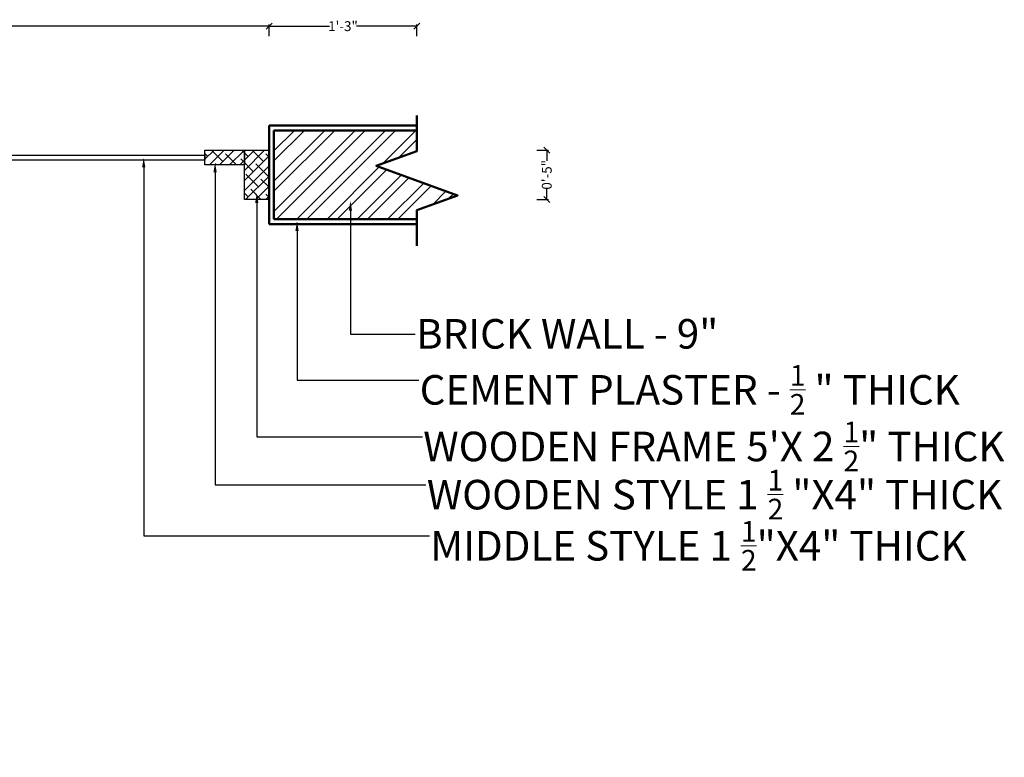
# Model space of a CAD drawing. Units: inches. Extents: x -54 to 163, y -154 to 48.
# Tile 2 of 3: x 30 to 129, y -154 to -79. Entities that reach past the tile are written whole.
import ezdxf
from ezdxf import colors
from ezdxf.entities.mleader import LeaderData, LeaderLine
from ezdxf.math import Vec2, Vec3

# ---------------------------------------------------------------- set-up
doc = ezdxf.new("R2010")
doc.units = ezdxf.units.IN
doc.header["$MEASUREMENT"] = 0
for name, color, linetype, lineweight in [('A-ANNO-DIMS', 2, 'Continuous', 18), ('A-ANNO-TEXT', 3, 'Continuous', 18), ('A-GLAZ', 4, 'Continuous', 25), ('A-GLAZ-PATT', 9, 'Continuous', 13), ('A-WALL', 7, 'Continuous', 50), ('A-WALL-PATT', 8, 'Continuous', 18)]:
    doc.layers.add(name, color=color, linetype=linetype, lineweight=lineweight)
doc.styles.get("Standard").update_dxf_attribs({"font": 'arial.ttf'})
doc.dimstyles.get("Standard").update_dxf_attribs({"dimtxt": 1, "dimasz": 0.6, "dimexe": 0.18, "dimexo": 0.0625, "dimgap": 0.09, "dimtad": 0, "dimdec": 1, "dimzin": 0, "dimdsep": 46, "dimlunit": 4, "dimtxsty": 'Standard', "dimblk": 'OBLIQUE', "dimcen": 0.09, "dimadec": 0, "dimazin": 0, "dimtfac": 1, "dimtdec": 1, "dimtofl": 0, "dimtmove": 0, "dimatfit": 3, "dimfxl": 1, "dimfxlon": 1, "dimtolj": 1, "dimtzin": 0, "dimarcsym": 0})

# ---------------------------------------------------------------- blocks, each defined once
blk = doc.blocks.new('_Oblique')
at = {"color": 0, "linetype": 'ByBlock', "lineweight": -2}
blk.add_line((-0.5, -0.5), (0.5, 0.5), dxfattribs=at)
blk = doc.blocks.new('*D34')
at = {"layer": 'A-ANNO-DIMS', "color": 0, "lineweight": -2, "transparency": 16777216}
for p, q in [((-24.085, -80.576), (-24.085, -79.396)), ((-24.085, -79.576), (13.993, -79.576)), ((54.915, -79.576), (16.837, -79.576)), ((54.915, -80.576), (54.915, -79.396))]:
    blk.add_line(p, q, dxfattribs=at)
at = {"layer": 'Defpoints', "color": 0, "transparency": 16777216}
for p in [(54.915, -79.576), (-24.085, -89.654), (54.915, -89.654)]:
    blk.add_point(p, dxfattribs=at)
at = {"layer": 'A-ANNO-DIMS', "color": 0, "lineweight": -2, "transparency": 16777216, "xscale": 0.6, "yscale": 0.6, "zscale": 0.6, "rotation": 180}
blk.add_blockref('_Oblique', (-24.085, -79.576), dxfattribs=at)
at = {"layer": 'A-ANNO-DIMS', "color": 0, "lineweight": -2, "transparency": 16777216, "xscale": 0.6, "yscale": 0.6, "zscale": 0.6}
blk.add_blockref('_Oblique', (54.915, -79.576), dxfattribs=at)
at = {"layer": 'A-ANNO-DIMS', "color": 0, "transparency": 16777216, "insert": (15.415, -79.576), "char_height": 1, "attachment_point": 5}
blk.add_mtext('\\A1;6\'-7"', dxfattribs=at)
blk = doc.blocks.new('*D35')
at = {"layer": 'A-ANNO-DIMS', "color": 0, "lineweight": -2, "transparency": 16777216}
for p, q in [((54.915, -80.576), (54.915, -79.396)), ((54.915, -79.576), (61.043, -79.576)), ((69.915, -79.576), (63.787, -79.576)), ((69.915, -80.576), (69.915, -79.396))]:
    blk.add_line(p, q, dxfattribs=at)
at = {"layer": 'Defpoints', "color": 0, "transparency": 16777216}
for p in [(69.915, -79.576), (54.915, -89.654), (69.915, -89.654)]:
    blk.add_point(p, dxfattribs=at)
at = {"layer": 'A-ANNO-DIMS', "color": 0, "lineweight": -2, "transparency": 16777216, "xscale": 0.6, "yscale": 0.6, "zscale": 0.6, "rotation": 180}
blk.add_blockref('_Oblique', (54.915, -79.576), dxfattribs=at)
at = {"layer": 'A-ANNO-DIMS', "color": 0, "lineweight": -2, "transparency": 16777216, "xscale": 0.6, "yscale": 0.6, "zscale": 0.6}
blk.add_blockref('_Oblique', (69.915, -79.576), dxfattribs=at)
at = {"layer": 'A-ANNO-DIMS', "color": 0, "transparency": 16777216, "insert": (62.415, -79.576), "char_height": 1, "attachment_point": 5}
blk.add_mtext('\\A1;1\'-3"', dxfattribs=at)
blk = doc.blocks.new('*D41')
at = {"layer": 'A-ANNO-DIMS', "color": 0, "lineweight": -2, "transparency": 16777216}
for p, q in [((-51.256, -89.654), (-52.436, -89.654)), ((-52.256, -89.654), (-52.256, -92.154)), ((-51.256, -92.154), (-52.436, -92.154)), ((-52.256, -92.154), (-52.256, -92.754))]:
    blk.add_line(p, q, dxfattribs=at)
at = {"layer": 'Defpoints', "color": 0, "transparency": 16777216}
for p in [(54.915, -89.654), (-52.256, -92.154), (52.415, -92.154)]:
    blk.add_point(p, dxfattribs=at)
at = {"layer": 'A-ANNO-DIMS', "color": 0, "lineweight": -2, "transparency": 16777216, "xscale": 0.6, "yscale": 0.6, "zscale": 0.6}
for p, rotation in [((-52.256, -89.654), 90), ((-52.256, -92.154), 270)]:
    blk.add_blockref('_Oblique', p, dxfattribs=dict(at, rotation=rotation))
at = {"layer": 'A-ANNO-DIMS', "color": 0, "transparency": 16777216, "insert": (-52.256, -95.339), "char_height": 1, "attachment_point": 5, "rotation": 90}
blk.add_mtext('\\A1;0\'-2 1/2"', dxfattribs=at)
blk = doc.blocks.new('*D42')
at = {"layer": 'A-ANNO-DIMS', "color": 0, "lineweight": -2, "transparency": 16777216}
for p, q in [((82.086, -92.154), (83.266, -92.154)), ((83.086, -92.154), (83.086, -93.235)), ((83.086, -97.154), (83.086, -96.073)), ((82.086, -97.154), (83.266, -97.154))]:
    blk.add_line(p, q, dxfattribs=at)
at = {"layer": 'Defpoints', "color": 0, "transparency": 16777216}
for p in [(-24.085, -92.154), (-24.085, -97.154), (83.086, -97.154)]:
    blk.add_point(p, dxfattribs=at)
at = {"layer": 'A-ANNO-DIMS', "color": 0, "lineweight": -2, "transparency": 16777216, "xscale": 0.6, "yscale": 0.6, "zscale": 0.6}
for p, rotation in [((83.086, -92.154), 90), ((83.086, -97.154), 270)]:
    blk.add_blockref('_Oblique', p, dxfattribs=dict(at, rotation=rotation))
at = {"layer": 'A-ANNO-DIMS', "color": 0, "transparency": 16777216, "insert": (83.086, -94.654), "char_height": 1, "attachment_point": 5, "rotation": 90}
blk.add_mtext('\\A1;0\'-5"', dxfattribs=at)

msp = doc.modelspace()

# ---------------------------------------------------------------- hatches: boundary and pattern name
at = {"layer": 'A-GLAZ-PATT'}
h = msp.add_hatch(dxfattribs=at)
h.set_pattern_fill('ANSI38', color=256, scale=5.8)
h.paths.add_polyline_path([(54.915, -92.154), (52.415, -92.154), (52.415, -97.154), (54.915, -97.154)])
h.paths.add_polyline_path([(52.415, -92.154), (48.415, -92.154), (48.415, -93.654), (52.415, -93.654)])
h.paths.add_polyline_path([(17.415, -92.154), (13.415, -92.154), (13.415, -93.654), (17.415, -93.654)])
h.paths.add_polyline_path([(-21.585, -92.154), (-24.085, -92.154), (-24.085, -97.154), (-21.585, -97.154)])
h.paths.add_polyline_path([(-17.585, -92.154), (-21.585, -92.154), (-21.585, -93.654), (-17.585, -93.654)])
at = {"layer": 'A-WALL-PATT'}
h = msp.add_hatch(dxfattribs=at)
h.set_pattern_fill('ANSI32', color=256, scale=5.8)
h.paths.add_polyline_path([(65.794, -93.742), (69.915, -92.242), (69.915, -90.154), (55.415, -90.154), (55.415, -99.154), (69.915, -99.154), (69.915, -98.242), (74.036, -96.742)])
h.paths.add_polyline_path([(-24.585, -90.154), (-39.085, -90.154), (-39.085, -92.242), (-34.964, -93.742), (-43.206, -96.742), (-39.085, -98.242), (-39.085, -99.154), (-24.585, -99.154)])

# ---------------------------------------------------------------- linework, layer by layer
at = {"layer": 'A-GLAZ'}
for points in [[(48.415, -92.654), (48.415, -93.154), (17.415, -93.154), (17.415, -92.654)], [(52.415, -92.154), (52.415, -93.654), (48.415, -93.654), (48.415, -92.154)], [(54.915, -92.154), (54.915, -97.154), (52.415, -97.154), (52.415, -92.154)]]:
    msp.add_lwpolyline(points, close=True, dxfattribs=at)
at = {"layer": 'A-WALL'}
for p, q in [((69.915, -89.654), (54.915, -89.654)), ((54.915, -89.654), (54.915, -99.654)), ((69.915, -90.154), (55.415, -90.154)), ((55.415, -90.154), (55.415, -99.154)), ((69.915, -99.654), (54.915, -99.654)), ((69.915, -99.154), (55.415, -99.154))]:
    msp.add_line(p, q, dxfattribs=at)
msp.add_lwpolyline([(69.915, -88.626), (69.915, -92.242), (65.794, -93.742), (74.036, -96.742), (69.915, -98.242), (69.915, -101.857)], dxfattribs=at)

# ---------------------------------------------------------------- dimensions: what is measured, and where the dimension line sits
at = {"layer": 'A-ANNO-DIMS'}
for base, p1, p2, picture, middle in [((54.915, -79.576), (-24.085, -89.654), (54.915, -89.654), '*D34', (15.415, -79.576)), ((69.915, -79.576), (54.915, -89.654), (69.915, -89.654), '*D35', (62.415, -79.576))]:
    dim = msp.add_linear_dim(base=base, p1=p1, p2=p2, dimstyle='Standard', override={"dimdec": 1, "dimlfac": 1, "dimrnd": 0, "dimzin": 1, "dimdsep": 46, "dimlunit": 4, "dimfrac": 2}, dxfattribs=at)
    dim.commit()
    dim.dimension.update_dxf_attribs({"geometry": picture, "text_midpoint": middle})
for base, p1, p2, picture, middle in [((-52.256, -92.154), (54.915, -89.654), (52.415, -92.154), '*D41', (-52.256, -95.339)), ((83.086, -97.154), (-24.085, -92.154), (-24.085, -97.154), '*D42', (83.086, -94.654))]:
    dim = msp.add_linear_dim(base=base, p1=p1, p2=p2, angle=90, dimstyle='Standard', override={"dimdec": 1, "dimlfac": 1, "dimrnd": 0, "dimzin": 1, "dimdsep": 46, "dimlunit": 4, "dimfrac": 2}, dxfattribs=at)
    dim.commit()
    dim.dimension.update_dxf_attribs({"geometry": picture, "text_midpoint": middle})

# ---------------------------------------------------------------- leaders
at = {"layer": 'A-ANNO-TEXT'}
ml = msp.add_multileader_mtext('Standard', dxfattribs=at)
ml.set_content('\\A1;MIDDLE STYLE 1 {\\H0.7x;\\S1/2;}"X4" THICK', color=256)
ml.set_leader_properties()
ml.build(insert=Vec2(0, 0))
ml.multileader.update_dxf_attribs({"dogleg_length": 0.36, "arrow_head_size": 1})
ctx = ml.context
ctx.base_point, ctx.char_height, ctx.arrow_head_size, ctx.landing_gap_size, ctx.plane_origin = Vec3(71.187, -131.294), 3, 1, 0.09, Vec3(42.201, -92.906)
notes = []
notes.append((ctx, [(0, (1, 1, 0), (70.827, -131.294), (1, 0), 0.36, [(0, [(42.201, -92.906), (42.201, -131.294)], 0, [])])]))
ctx.mtext.insert, ctx.mtext.flow_direction = Vec3(71.277, -129.769), 5
ml = msp.add_multileader_mtext('Standard', dxfattribs=at)
ml.set_content('\\A1;WOODEN STYLE 1 {\\H0.7x;\\S1/2;} "X4" THICK', color=256)
ml.set_leader_properties()
ml.build(insert=Vec2(0, 0))
ml.multileader.update_dxf_attribs({"dogleg_length": 0.36, "arrow_head_size": 1})
ctx = ml.context
ctx.base_point, ctx.char_height, ctx.arrow_head_size, ctx.landing_gap_size, ctx.plane_origin = Vec3(70.827, -126.107), 3, 1, 0.09, Vec3(49.439, -93.397)
notes.append((ctx, [(0, (1, 1, 0), (70.467, -126.107), (1, 0), 0.36, [(0, [(49.439, -93.397), (49.439, -126.107)], 0, [])])]))
ctx.mtext.insert, ctx.mtext.flow_direction = Vec3(70.917, -124.581), 5
ml = msp.add_multileader_mtext('Standard', dxfattribs=at)
ml.set_content('\\A1;WOODEN FRAME 5\'X 2 {\\H0.7x;\\S1/2;}" THICK', color=256)
ml.set_leader_properties()
ml.build(insert=Vec2(0, 0))
ml.multileader.update_dxf_attribs({"dogleg_length": 0.36, "arrow_head_size": 1})
ctx = ml.context
ctx.base_point, ctx.char_height, ctx.arrow_head_size, ctx.landing_gap_size, ctx.plane_origin = Vec3(70.467, -121.222), 3, 1, 0.09, Vec3(53.665, -96.506)
notes.append((ctx, [(0, (1, 1, 0), (70.107, -121.222), (1, 0), 0.36, [(0, [(53.665, -96.506), (53.665, -121.222)], 0, [])])]))
ctx.mtext.insert, ctx.mtext.flow_direction = Vec3(70.557, -119.696), 5
ml = msp.add_multileader_mtext('Standard', dxfattribs=at)
ml.set_content('BRICK WALL - 9"', color=256)
ml.set_leader_properties()
ml.build(insert=Vec2(0, 0))
ml.multileader.update_dxf_attribs({"dogleg_length": 0.36, "arrow_head_size": 1})
ctx = ml.context
ctx.base_point, ctx.char_height, ctx.arrow_head_size, ctx.landing_gap_size, ctx.plane_origin = Vec3(69.747, -110.815), 3, 1, 0.09, Vec3(63.168, -97.29)
notes.append((ctx, [(0, (1, 1, 0), (69.387, -110.815), (1, 0), 0.36, [(0, [(63.168, -97.29), (63.168, -110.815)], 0, [])])]))
ctx.mtext.insert, ctx.mtext.flow_direction = Vec3(69.837, -109.289), 5
ml = msp.add_multileader_mtext('Standard', dxfattribs=at)
ml.set_content('\\A1;CEMENT PLASTER - {\\H0.7x;\\S1/2;} " THICK', color=256)
ml.set_leader_properties()
ml.build(insert=Vec2(0, 0))
ml.multileader.update_dxf_attribs({"dogleg_length": 0.36, "arrow_head_size": 1})
ctx = ml.context
ctx.base_point, ctx.char_height, ctx.arrow_head_size, ctx.landing_gap_size, ctx.plane_origin = Vec3(70.107, -115.477), 3, 1, 0.09, Vec3(57.751, -99.343)
notes.append((ctx, [(0, (1, 1, 0), (69.747, -115.477), (1, 0), 0.36, [(0, [(57.751, -99.343), (57.751, -115.477)], 0, [])])]))
ctx.mtext.insert, ctx.mtext.flow_direction = Vec3(70.197, -113.951), 5
for ctx, leaders in notes:
    for number, flags, end, landing, length, lines in leaders:
        leader = LeaderData()
        leader.index, (leader.has_last_leader_line, leader.has_dogleg_vector, leader.attachment_direction) = number, flags
        leader.last_leader_point, leader.dogleg_vector, leader.dogleg_length = Vec3(end), Vec3(landing), length
        for number, points, colour, breaks in lines:
            line = LeaderLine()
            line.index, line.vertices, line.color, line.breaks = number, Vec3.list(points), colors.encode_raw_color(colour), breaks
            leader.lines.append(line)
        ctx.leaders.append(leader)

doc.saveas('drawing.dxf')
